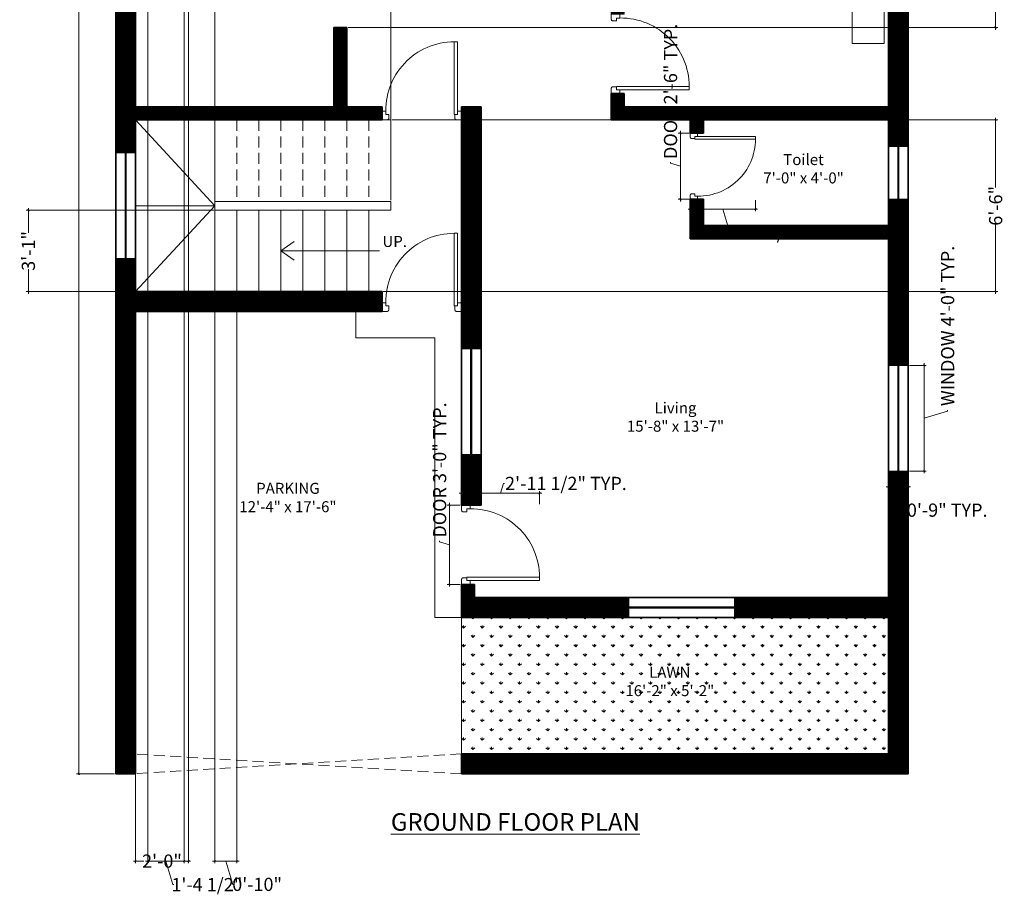
# Model space of a CAD drawing. Units: inches. Extents: x 111008 to 118198, y -138546 to -137723.
# Tile 3 of 4: x 117735 to 118183, y -138546 to -138144. Entities that reach past the tile are written whole.
import ezdxf

# ---------------------------------------------------------------- set-up
doc = ezdxf.new("R2010")
doc.units = ezdxf.units.IN
doc.header["$LTSCALE"] = 20
doc.header["$MEASUREMENT"] = 0
doc.header["$PDMODE"] = 3
doc.linetypes.add('HIDDEN', pattern=[0.375, 0.25, -0.125])
for name, color, linetype, lineweight in [('A-ANNO-DIMS', 2, 'Continuous', 18), ('A-ANNO-TEXT', 7, 'Continuous', 18), ('A-AREA-IDEN', 7, 'Continuous', 18), ('A-DOOR', 181, 'Continuous', 18), ('A-DOOR-HIDN', 1, 'HIDDEN', 13), ('A-FLOR-CASE', 181, 'Continuous', 18), ('A-FLOR-STRS', 181, 'Continuous', 18), ('A-FLOR-STRS-HIDN', 181, 'HIDDEN', 13), ('ele', 6, 'Continuous', 20), ('furn', 181, 'Continuous', 15), ('FURNITURE', 8, 'Continuous', 15), ('L-PVMT', 181, 'Continuous', 18), ('walls', 7, 'Continuous', 35), ('WIN', 181, 'Continuous', 18)]:
    doc.layers.add(name, color=color, linetype=linetype, lineweight=lineweight)
doc.layers.add('A-WALL-PATT', color=251, linetype='Continuous', lineweight=9, true_color=0x636466)
doc.layers.add('L-PLNT-PATT', color=114, linetype='Continuous', lineweight=9, true_color=0x139b48)
doc.styles.add('vn1', font='arial.ttf', dxfattribs={"height": 6})
doc.dimstyles.new('vn1', dxfattribs={"dimtxt": 6, "dimasz": 1, "dimexe": 1, "dimexo": 0.5, "dimgap": 0.25, "dimtad": 0, "dimdec": 1, "dimzin": 3, "dimdsep": 46, "dimlunit": 4, "dimtxsty": 'vn1', "dimblk": 'ARCHTICK', "dimcen": 0, "dimdle": 1, "dimclrd": 8, "dimclre": 8, "dimclrt": 7, "dimadec": 0, "dimazin": 0, "dimtfac": 0.75, "dimtdec": 1, "dimtofl": 0, "dimtmove": 1, "dimatfit": 3, "dimfxl": 1, "dimtolj": 1, "dimtzin": 0, "dimlwd": -1, "dimlwe": -1, "dimarcsym": 0})

# ---------------------------------------------------------------- blocks, each defined once
blk = doc.blocks.new('_ArchTick')
at = {"color": 0, "linetype": 'ByBlock', "const_width": 0.15}
blk.add_lwpolyline([(-0.5, -0.5), (0.5, 0.5)], dxfattribs=at)
blk = doc.blocks.new('*D4')
at = {"layer": 'A-ANNO-DIMS', "color": 0, "transparency": 16777216}
for p, q in [((117778.41, -137766.56), (117761.13, -137766.56)), ((117762.13, -137766.06), (117762.13, -138115.99)), ((117762.13, -138487.06), (117762.13, -138137.13)), ((117778.41, -138486.56), (117761.13, -138486.56))]:
    blk.add_line(p, q, dxfattribs=at)
at = {"layer": 'Defpoints', "color": 0, "transparency": 16777216}
for p in [(117762.13, -137766.56), (117778.91, -137766.56), (117778.91, -138486.56)]:
    blk.add_point(p, dxfattribs=at)
at = {"layer": 'A-ANNO-DIMS', "color": 0, "transparency": 16777216}
for p, rotation in [((117762.13, -137766.56), 90), ((117762.13, -138486.56), 270)]:
    blk.add_blockref('_ArchTick', p, dxfattribs=dict(at, rotation=rotation))
at = {"layer": 'A-ANNO-DIMS', "color": 0, "transparency": 16777216, "insert": (117762.13, -138126.56), "char_height": 6, "attachment_point": 5, "rotation": 90, "style": 'vn1'}
blk.add_mtext('\\A1;60\'-0"', dxfattribs=at)
blk = doc.blocks.new('39 door')
at = {"layer": 'ele'}
blk.add_lwpolyline([(-17.62, 38.46), (-17.62, 2.69), (-16, 2.69), (-16, 38.46)], close=True, dxfattribs=at)
at = {"layer": 'furn'}
for points in [[(-16.87, 0), (-19.5, 0), (-19.5, 0), (-19.5, 4.31), (-17.62, 4.31), (-17.62, 2.69), (-16.27, 2.69), (-16.27, 0.6), (-16.42, 0.6), (-16.42, 0.45, -0.414214), (-16.72, 0.15), (-16.87, 0.15)], [(16.87, 0), (19.5, 0), (19.5, 0), (19.5, 4.31), (17.62, 4.31), (17.62, 2.69), (16.27, 2.69), (16.27, 0.6), (16.42, 0.6), (16.42, 0.45, 0.414214), (16.72, 0.15), (16.87, 0.15)]]:
    blk.add_lwpolyline(points, format="xyb", close=True, dxfattribs=at)
at = {"layer": 'WIN', "ltscale": 0.25}
blk.add_arc((-16.03, 4.75), 33.71, 356.5003, 89.9437, dxfattribs=at)
blk = doc.blocks.new('WIN-48IN')
at = {"ltscale": 0.5}
for p, q in [((0, 48), (0, 0)), ((9, 48), (9, 0))]:
    blk.add_line(p, q, dxfattribs=at)
for p, q in [((0, 48), (9, 48)), ((0, 0), (9, 0))]:
    blk.add_line(p, q)
at = {"ltscale": 0.5, "const_width": 1}
blk.add_lwpolyline([(4.49, 48), (4.49, 0)], dxfattribs=at)
blk = doc.blocks.new('WIN-24IN')
at = {"ltscale": 0.5}
for p, q in [((0, 24), (0, 0)), ((9, 24), (9, 0))]:
    blk.add_line(p, q, dxfattribs=at)
for p, q in [((0, 24), (9, 24)), ((0, 0), (9, 0))]:
    blk.add_line(p, q)
at = {"ltscale": 0.5, "const_width": 1}
blk.add_lwpolyline([(4.49, 24), (4.49, 0)], dxfattribs=at)
blk = doc.blocks.new('BEDSIDE-TABLE')
blk.add_lwpolyline([(0, 16.95), (0, 0), (14.43, 0), (14.43, 16.95)], close=True)
blk = doc.blocks.new('*D11')
at = {"layer": 'A-ANNO-DIMS', "color": 8, "transparency": 16777216}
for p, q in [((117930.51, -138401.56), (117930.51, -138363.56)), ((117935.41, -138364.56), (117929.51, -138364.56)), ((117926.03, -138381.21), (117926.03, -138380.71)), ((117930.51, -138382.56), (117926.03, -138381.21)), ((117935.41, -138400.56), (117929.51, -138400.56))]:
    blk.add_line(p, q, dxfattribs=at)
at = {"layer": 'Defpoints', "color": 0, "transparency": 16777216}
for p in [(117930.51, -138364.56), (117935.91, -138364.56), (117935.91, -138400.56)]:
    blk.add_point(p, dxfattribs=at)
at = {"layer": 'A-ANNO-DIMS', "color": 8, "transparency": 16777216}
for p, rotation in [((117930.51, -138364.56), 90), ((117930.51, -138400.56), 270)]:
    blk.add_blockref('_ArchTick', p, dxfattribs=dict(at, rotation=rotation))
at = {"layer": 'A-ANNO-DIMS', "color": 7, "transparency": 16777216, "insert": (117926.03, -138348.59), "char_height": 6, "attachment_point": 5, "rotation": 90, "style": 'vn1'}
blk.add_mtext('\\A1;DOOR 3\'-0" TYP.', dxfattribs=at)
blk = doc.blocks.new('*D12')
at = {"layer": 'A-ANNO-DIMS', "color": 8, "transparency": 16777216}
for p, q in [((117953.66, -138359.16), (117955, -138354.68)), ((117955, -138354.68), (117955.5, -138354.68)), ((117934.91, -138359.16), (117972.41, -138359.16)), ((117935.91, -138364.06), (117935.91, -138358.16)), ((117971.41, -138364.06), (117971.41, -138358.16))]:
    blk.add_line(p, q, dxfattribs=at)
at = {"layer": 'Defpoints', "color": 0, "transparency": 16777216}
for p in [(117971.41, -138359.16), (117935.91, -138364.56), (117971.41, -138364.56)]:
    blk.add_point(p, dxfattribs=at)
at = {"layer": 'A-ANNO-DIMS', "color": 8, "transparency": 16777216, "rotation": 180}
blk.add_blockref('_ArchTick', (117935.91, -138359.16), dxfattribs=at)
at = {"layer": 'A-ANNO-DIMS', "color": 8, "transparency": 16777216}
blk.add_blockref('_ArchTick', (117971.41, -138359.16), dxfattribs=at)
at = {"layer": 'A-ANNO-DIMS', "color": 7, "transparency": 16777216, "insert": (117983.41, -138354.68), "char_height": 6, "attachment_point": 5, "style": 'vn1'}
blk.add_mtext('\\A1;2\'-11 1/2" TYP.', dxfattribs=at)
blk = doc.blocks.new('*D13')
at = {"layer": 'A-ANNO-DIMS', "color": 8, "transparency": 16777216}
for p, q in [((118039.41, -138195.56), (118034.41, -138195.55)), ((118035.41, -138194.55), (118035.39, -138226.55)), ((118030.92, -138209.21), (118030.92, -138208.71)), ((118035.4, -138210.55), (118030.92, -138209.21)), ((118039.39, -138225.56), (118034.39, -138225.55))]:
    blk.add_line(p, q, dxfattribs=at)
at = {"layer": 'Defpoints', "color": 0, "transparency": 16777216}
for p in [(118039.91, -138195.56), (118035.39, -138225.55), (118039.89, -138225.56)]:
    blk.add_point(p, dxfattribs=at)
at = {"layer": 'A-ANNO-DIMS', "color": 8, "transparency": 16777216}
for p, rotation in [((118035.41, -138195.55), 89.96632877380524), ((118035.39, -138225.55), 269.9663287738052)]:
    blk.add_blockref('_ArchTick', p, dxfattribs=dict(at, rotation=rotation))
at = {"layer": 'A-ANNO-DIMS', "color": 7, "transparency": 16777216, "insert": (118030.94, -138176.58), "char_height": 6, "attachment_point": 5, "rotation": 89.9663, "style": 'vn1'}
blk.add_mtext('\\A1;DOOR 2\'-6" TYP.', dxfattribs=at)
blk = doc.blocks.new('*D14')
at = {"layer": 'A-ANNO-DIMS', "color": 8, "transparency": 16777216}
for p, q in [((118038.89, -138230.06), (118070.47, -138230.08)), ((118039.89, -138226.06), (118039.89, -138231.06)), ((118054.68, -138230.07), (118057.88, -138240.75)), ((118069.48, -138226.07), (118069.47, -138231.07)), ((118057.88, -138240.75), (118058.38, -138240.75))]:
    blk.add_line(p, q, dxfattribs=at)
at = {"layer": 'Defpoints', "color": 0, "transparency": 16777216}
for p in [(118039.89, -138225.56), (118069.48, -138225.57), (118069.47, -138230.07)]:
    blk.add_point(p, dxfattribs=at)
at = {"layer": 'A-ANNO-DIMS', "color": 8, "transparency": 16777216}
for p, rotation in [((118039.89, -138230.06), 179.9663287737755), ((118069.47, -138230.07), 359.9663287737755)]:
    blk.add_blockref('_ArchTick', p, dxfattribs=dict(at, rotation=rotation))
at = {"layer": 'A-ANNO-DIMS', "color": 7, "transparency": 16777216, "insert": (118083.96, -138240.77), "char_height": 6, "attachment_point": 5, "rotation": 359.9663, "style": 'vn1'}
blk.add_mtext('\\A1;2\'-5 1/2" TYP.', dxfattribs=at)
blk = doc.blocks.new('*D15')
at = {"layer": 'A-ANNO-DIMS', "color": 8, "transparency": 16777216}
for p, q in [((118139.41, -138301.06), (118147.11, -138301.06)), ((118146.11, -138350.06), (118146.11, -138300.06)), ((118146.11, -138325.06), (118156.8, -138321.85)), ((118156.8, -138321.85), (118156.8, -138321.35)), ((118139.41, -138349.06), (118147.11, -138349.06))]:
    blk.add_line(p, q, dxfattribs=at)
at = {"layer": 'Defpoints', "color": 0, "transparency": 16777216}
for p in [(118138.91, -138301.06), (118146.11, -138301.06), (118138.91, -138349.06)]:
    blk.add_point(p, dxfattribs=at)
at = {"layer": 'A-ANNO-DIMS', "color": 8, "transparency": 16777216}
for p, rotation in [((118146.11, -138301.06), 90), ((118146.11, -138349.06), 270)]:
    blk.add_blockref('_ArchTick', p, dxfattribs=dict(at, rotation=rotation))
at = {"layer": 'A-ANNO-DIMS', "color": 7, "transparency": 16777216, "insert": (118156.8, -138283.14), "char_height": 6, "attachment_point": 5, "rotation": 90, "style": 'vn1'}
blk.add_mtext('\\A1;WINDOW 4\'-0" TYP.', dxfattribs=at)
blk = doc.blocks.new('*D16')
at = {"layer": 'A-ANNO-DIMS', "color": 8, "transparency": 16777216}
for p, q in [((118129.91, -138349.56), (118129.91, -138357.26)), ((118138.91, -138349.56), (118138.91, -138357.26)), ((118128.91, -138356.26), (118139.91, -138356.26)), ((118134.41, -138356.26), (118137.58, -138366.82)), ((118137.58, -138366.82), (118138.08, -138366.82))]:
    blk.add_line(p, q, dxfattribs=at)
at = {"layer": 'Defpoints', "color": 0, "transparency": 16777216}
for p in [(118129.91, -138349.06), (118138.91, -138349.06), (118138.91, -138356.26)]:
    blk.add_point(p, dxfattribs=at)
at = {"layer": 'A-ANNO-DIMS', "color": 8, "transparency": 16777216, "rotation": 180}
blk.add_blockref('_ArchTick', (118129.91, -138356.26), dxfattribs=at)
at = {"layer": 'A-ANNO-DIMS', "color": 8, "transparency": 16777216}
blk.add_blockref('_ArchTick', (118138.91, -138356.26), dxfattribs=at)
at = {"layer": 'A-ANNO-DIMS', "color": 7, "transparency": 16777216, "insert": (118156.61, -138366.82), "char_height": 6, "attachment_point": 5, "style": 'vn1'}
blk.add_mtext('\\A1;0\'-9" TYP.', dxfattribs=at)
blk = doc.blocks.new('*D25')
at = {"layer": 'A-ANNO-DIMS', "color": 8, "transparency": 16777216}
for p, q in [((117787.91, -138184.06), (117787.91, -138527.26)), ((117811.91, -138184.06), (117811.91, -138527.26)), ((117786.91, -138526.26), (117791.63, -138526.26)), ((117812.91, -138526.26), (117808.18, -138526.26))]:
    blk.add_line(p, q, dxfattribs=at)
at = {"layer": 'Defpoints', "color": 0, "transparency": 16777216}
for p in [(117787.91, -138183.56), (117811.91, -138183.56), (117811.91, -138526.26)]:
    blk.add_point(p, dxfattribs=at)
at = {"layer": 'A-ANNO-DIMS', "color": 8, "transparency": 16777216, "rotation": 180}
blk.add_blockref('_ArchTick', (117787.91, -138526.26), dxfattribs=at)
at = {"layer": 'A-ANNO-DIMS', "color": 8, "transparency": 16777216}
blk.add_blockref('_ArchTick', (117811.91, -138526.26), dxfattribs=at)
at = {"layer": 'A-ANNO-DIMS', "color": 7, "transparency": 16777216, "insert": (117799.91, -138526.26), "char_height": 6, "attachment_point": 5, "style": 'vn1'}
blk.add_mtext('\\A1;2\'-0"', dxfattribs=at)
blk = doc.blocks.new('*D26')
at = {"layer": 'A-ANNO-DIMS', "color": 8, "transparency": 16777216}
for p, q in [((117884.41, -138063.56), (118179.61, -138063.56)), ((118178.61, -138062.56), (118178.61, -138097.36)), ((118178.61, -138148.56), (118178.61, -138113.76)), ((117884.41, -138147.56), (118179.61, -138147.56))]:
    blk.add_line(p, q, dxfattribs=at)
at = {"layer": 'Defpoints', "color": 0, "transparency": 16777216}
for p in [(117883.91, -138063.56), (117883.91, -138147.56), (118178.61, -138147.56)]:
    blk.add_point(p, dxfattribs=at)
at = {"layer": 'A-ANNO-DIMS', "color": 8, "transparency": 16777216}
for p, rotation in [((118178.61, -138063.56), 90), ((118178.61, -138147.56), 270)]:
    blk.add_blockref('_ArchTick', p, dxfattribs=dict(at, rotation=rotation))
at = {"layer": 'A-ANNO-DIMS', "color": 7, "transparency": 16777216, "insert": (118178.61, -138105.56), "char_height": 6, "attachment_point": 5, "rotation": 90, "style": 'vn1'}
blk.add_mtext('\\A1;7\'-0"', dxfattribs=at)
blk = doc.blocks.new('*D27')
at = {"layer": 'A-ANNO-DIMS', "color": 8, "transparency": 16777216}
for p, q in [((117793.41, -138135.94), (117793.41, -138527.26)), ((117809.91, -138135.94), (117809.91, -138527.26)), ((117792.41, -138526.26), (117810.91, -138526.26)), ((117801.66, -138526.26), (117804.86, -138536.94)), ((117804.86, -138536.94), (117805.36, -138536.94))]:
    blk.add_line(p, q, dxfattribs=at)
at = {"layer": 'Defpoints', "color": 0, "transparency": 16777216}
for p in [(117793.41, -138135.44), (117809.91, -138135.44), (117809.91, -138526.26)]:
    blk.add_point(p, dxfattribs=at)
at = {"layer": 'A-ANNO-DIMS', "color": 8, "transparency": 16777216, "rotation": 180}
blk.add_blockref('_ArchTick', (117793.41, -138526.26), dxfattribs=at)
at = {"layer": 'A-ANNO-DIMS', "color": 8, "transparency": 16777216}
blk.add_blockref('_ArchTick', (117809.91, -138526.26), dxfattribs=at)
at = {"layer": 'A-ANNO-DIMS', "color": 7, "transparency": 16777216, "insert": (117820.29, -138536.94), "char_height": 6, "attachment_point": 5, "style": 'vn1'}
blk.add_mtext('\\A1;1\'-4 1/2"', dxfattribs=at)
blk = doc.blocks.new('*D31')
at = {"layer": 'A-ANNO-DIMS', "color": 8, "transparency": 16777216}
for p, q in [((117823.91, -138268.06), (117823.91, -138527.26)), ((117833.91, -138268.06), (117833.91, -138527.26)), ((117822.91, -138526.26), (117834.91, -138526.26)), ((117828.91, -138526.26), (117832.08, -138536.82)), ((117832.08, -138536.82), (117832.58, -138536.82))]:
    blk.add_line(p, q, dxfattribs=at)
at = {"layer": 'Defpoints', "color": 0, "transparency": 16777216}
for p in [(117823.91, -138267.56), (117833.91, -138267.56), (117833.91, -138526.26)]:
    blk.add_point(p, dxfattribs=at)
at = {"layer": 'A-ANNO-DIMS', "color": 8, "transparency": 16777216, "rotation": 180}
blk.add_blockref('_ArchTick', (117823.91, -138526.26), dxfattribs=at)
at = {"layer": 'A-ANNO-DIMS', "color": 8, "transparency": 16777216}
blk.add_blockref('_ArchTick', (117833.91, -138526.26), dxfattribs=at)
at = {"layer": 'A-ANNO-DIMS', "color": 7, "transparency": 16777216, "insert": (117843.13, -138536.82), "char_height": 6, "attachment_point": 5, "style": 'vn1'}
blk.add_mtext('\\A1;0\'-10"', dxfattribs=at)
blk = doc.blocks.new('*D32')
at = {"layer": 'A-ANNO-DIMS', "color": 8, "transparency": 16777216}
for p, q in [((117739.21, -138229.56), (117739.21, -138240.83)), ((117823.41, -138230.56), (117738.21, -138230.56)), ((117739.21, -138268.56), (117739.21, -138257.28)), ((117823.41, -138267.56), (117738.21, -138267.56))]:
    blk.add_line(p, q, dxfattribs=at)
at = {"layer": 'Defpoints', "color": 0, "transparency": 16777216}
for p in [(117739.21, -138230.56), (117823.91, -138230.56), (117823.91, -138267.56)]:
    blk.add_point(p, dxfattribs=at)
at = {"layer": 'A-ANNO-DIMS', "color": 8, "transparency": 16777216}
for p, rotation in [((117739.21, -138230.56), 90), ((117739.21, -138267.56), 270)]:
    blk.add_blockref('_ArchTick', p, dxfattribs=dict(at, rotation=rotation))
at = {"layer": 'A-ANNO-DIMS', "color": 7, "transparency": 16777216, "insert": (117739.21, -138249.06), "char_height": 6, "attachment_point": 5, "rotation": 90, "style": 'vn1'}
blk.add_mtext('\\A1;3\'-1"', dxfattribs=at)
blk = doc.blocks.new('*D33')
at = {"layer": 'A-ANNO-DIMS', "color": 8, "transparency": 16777216}
for p, q in [((117786.91, -137726.86), (117797.68, -137726.86)), ((117787.91, -138228.06), (117787.91, -137725.86)), ((117824.91, -137726.86), (117814.13, -137726.86)), ((117823.91, -138228.06), (117823.91, -137725.86))]:
    blk.add_line(p, q, dxfattribs=at)
at = {"layer": 'Defpoints', "color": 0, "transparency": 16777216}
for p in [(117823.91, -137726.86), (117787.91, -138228.56), (117823.91, -138228.56)]:
    blk.add_point(p, dxfattribs=at)
at = {"layer": 'A-ANNO-DIMS', "color": 8, "transparency": 16777216, "rotation": 180}
blk.add_blockref('_ArchTick', (117787.91, -137726.86), dxfattribs=at)
at = {"layer": 'A-ANNO-DIMS', "color": 8, "transparency": 16777216}
blk.add_blockref('_ArchTick', (117823.91, -137726.86), dxfattribs=at)
at = {"layer": 'A-ANNO-DIMS', "color": 7, "transparency": 16777216, "insert": (117805.91, -137726.86), "char_height": 6, "attachment_point": 5, "style": 'vn1'}
blk.add_mtext('\\A1;3\'-0"', dxfattribs=at)
blk = doc.blocks.new('*D34')
at = {"layer": 'A-ANNO-DIMS', "color": 8, "transparency": 16777216}
for p, q in [((117822.91, -137726.86), (117855.67, -137726.86)), ((117823.91, -138226.06), (117823.91, -137725.86)), ((117904.91, -137726.86), (117872.15, -137726.86)), ((117903.91, -138226.06), (117903.91, -137725.86))]:
    blk.add_line(p, q, dxfattribs=at)
at = {"layer": 'Defpoints', "color": 0, "transparency": 16777216}
for p in [(117903.91, -137726.86), (117823.91, -138226.56), (117903.91, -138226.56)]:
    blk.add_point(p, dxfattribs=at)
at = {"layer": 'A-ANNO-DIMS', "color": 8, "transparency": 16777216, "rotation": 180}
blk.add_blockref('_ArchTick', (117823.91, -137726.86), dxfattribs=at)
at = {"layer": 'A-ANNO-DIMS', "color": 8, "transparency": 16777216}
blk.add_blockref('_ArchTick', (117903.91, -137726.86), dxfattribs=at)
at = {"layer": 'A-ANNO-DIMS', "color": 7, "transparency": 16777216, "insert": (117863.91, -137726.86), "char_height": 6, "attachment_point": 5, "style": 'vn1'}
blk.add_mtext('\\A1;6\'-8"', dxfattribs=at)
blk = doc.blocks.new('*D35')
at = {"layer": 'A-ANNO-DIMS', "color": 8, "transparency": 16777216}
for p, q in [((117904.41, -138189.56), (118179.61, -138189.56)), ((118178.61, -138188.56), (118178.61, -138220.32)), ((118178.61, -138268.56), (118178.61, -138236.8)), ((117900.41, -138267.56), (118179.61, -138267.56))]:
    blk.add_line(p, q, dxfattribs=at)
at = {"layer": 'Defpoints', "color": 0, "transparency": 16777216}
for p in [(117903.91, -138189.56), (118178.61, -138189.56), (117899.91, -138267.56)]:
    blk.add_point(p, dxfattribs=at)
at = {"layer": 'A-ANNO-DIMS', "color": 8, "transparency": 16777216}
for p, rotation in [((118178.61, -138189.56), 90), ((118178.61, -138267.56), 270)]:
    blk.add_blockref('_ArchTick', p, dxfattribs=dict(at, rotation=rotation))
at = {"layer": 'A-ANNO-DIMS', "color": 7, "transparency": 16777216, "insert": (118178.61, -138228.56), "char_height": 6, "attachment_point": 5, "rotation": 90, "style": 'vn1'}
blk.add_mtext('\\A1;6\'-6"', dxfattribs=at)

msp = doc.modelspace()

# ---------------------------------------------------------------- hatches: boundary and pattern name
at = {"layer": 'A-WALL-PATT'}
h = msp.add_hatch(dxfattribs=at)
h.set_pattern_fill('ANSI31', color=256)
h.paths.add_polyline_path([(117829.91, -137766.56), (117778.91, -137766.56), (117778.91, -137919.56), (117787.91, -137919.56), (117787.91, -137865.56), (117826.91, -137865.56), (117826.91, -137859.56), (117787.91, -137859.56), (117787.91, -137775.56), (117829.91, -137775.56)])
h.paths.add_polyline_path([(117865.91, -137766.56), (117853.91, -137766.56), (117853.91, -137775.56), (117859.91, -137775.56), (117859.91, -137859.56), (117856.91, -137859.56), (117856.91, -137865.56), (117868.91, -137865.56), (117868.91, -137861.58), (117868.91, -137859.56), (117865.91, -137859.56)])
h.paths.add_polyline_path([(118099.91, -137766.56), (118051.91, -137766.56), (118051.91, -137859.56), (118048.91, -137859.56), (118048.91, -137865.56), (118060.91, -137865.56), (118060.91, -137862.24), (118060.91, -137859.56), (118057.91, -137859.56), (118057.91, -137775.56), (118099.91, -137775.56)])
h.paths.add_polyline_path([(118138.91, -137766.56), (118123.91, -137766.56), (118123.91, -137775.56), (118129.91, -137775.56), (118129.91, -137859.56), (118090.91, -137859.56), (118090.91, -137865.56), (118129.91, -137865.56), (118129.91, -137919.56), (118138.91, -137919.56)])
h.paths.add_polyline_path([(118138.91, -137967.56), (118129.91, -137967.56), (118129.91, -138021.56), (118003.91, -138021.56), (118003.91, -138141.56), (118007.88, -138141.56), (118009.91, -138141.56), (118009.91, -138027.56), (118129.91, -138027.56), (118129.91, -138081.56), (118138.91, -138081.56)])
h.paths.add_polyline_path([(118012.91, -137861.58), (118012.91, -137859.56), (117904.91, -137859.56), (117904.91, -137865.56), (117960.91, -137865.56), (117960.91, -138021.56), (117954.91, -138021.56), (117954.91, -138027.56), (117967.91, -138027.56), (117967.91, -138023.58), (117967.91, -138021.56), (117966.91, -138021.56), (117966.91, -137865.56), (118012.91, -137865.56)])
h.paths.add_polyline_path([(117787.91, -138027.56), (117877.91, -138027.56), (117877.91, -138063.56), (117883.91, -138063.56), (117883.91, -138027.56), (117918.91, -138027.56), (117918.91, -138023.58), (117918.91, -138021.56), (117787.91, -138021.56), (117787.91, -137967.56), (117778.91, -137967.56), (117778.91, -138081.56), (117787.91, -138081.56)])
h.paths.add_polyline_path([(117787.91, -138129.56), (117778.91, -138129.56), (117778.91, -138204.56), (117787.91, -138204.56), (117787.91, -138189.56), (117899.91, -138189.56), (117899.91, -138185.58), (117899.91, -138183.56), (117883.91, -138183.56), (117883.91, -138147.56), (117877.91, -138147.56), (117877.91, -138183.56), (117787.91, -138183.56)])
h.paths.add_polyline_path([(118138.91, -138129.56), (118129.91, -138129.56), (118129.91, -138183.56), (118009.91, -138183.56), (118009.91, -138177.56), (118003.91, -138177.56), (118003.91, -138189.56), (118039.91, -138189.56), (118039.91, -138195.56), (118045.91, -138195.56), (118045.91, -138189.56), (118129.91, -138189.56), (118129.91, -138201.56), (118138.91, -138201.56)])
h.paths.add_polyline_path([(118138.91, -138225.56), (118129.91, -138225.56), (118129.91, -138237.56), (118045.91, -138237.56), (118045.91, -138225.56), (118043.2, -138225.56), (118043.2, -138225.56), (118039.91, -138225.56), (118039.91, -138243.56), (118129.91, -138243.56), (118129.91, -138301.06), (118138.91, -138301.06)])
h.paths.add_polyline_path([(117944.91, -138183.56), (117935.91, -138183.56), (117935.91, -138293.56), (117944.91, -138293.56)])
h.paths.add_polyline_path([(117899.91, -138267.56), (117787.91, -138267.56), (117787.91, -138252.56), (117778.91, -138252.56), (117778.91, -138486.56), (117787.91, -138486.56), (117787.91, -138276.56), (117899.91, -138276.56), (117899.91, -138272.58)])
h.paths.add_polyline_path([(117944.91, -138341.56), (117935.91, -138341.56), (117935.91, -138364.56), (117939.88, -138364.56), (117944.91, -138364.56)])
h.paths.add_polyline_path([(118011.91, -138406.56), (117941.91, -138406.56), (117941.91, -138400.56), (117935.91, -138400.56), (117935.91, -138415.56), (118011.91, -138415.56)], flags=17)
h.paths.add_polyline_path([(118138.91, -138349.06), (118129.91, -138349.06), (118129.91, -138406.56), (118059.91, -138406.56), (118059.91, -138415.56), (118129.91, -138415.56), (118129.91, -138477.56), (117935.91, -138477.56), (117935.91, -138486.56), (118138.91, -138486.56)])
at = {"layer": 'L-PLNT-PATT'}
h = msp.add_hatch(dxfattribs=at)
h.set_pattern_fill('GRASS', color=256, scale=6)
h.paths.add_polyline_path([(118129.91, -138415.56), (117935.91, -138415.56), (117935.91, -138477.56), (118129.91, -138477.56)])

# ---------------------------------------------------------------- linework, layer by layer
at = {"layer": 'A-DOOR-HIDN'}
for p, q in [((117935.91, -138486.56), (117787.91, -138477.56)), ((117935.91, -138477.56), (117787.91, -138486.56))]:
    msp.add_line(p, q, dxfattribs=at)
at = {"layer": 'A-FLOR-CASE'}
msp.add_line((117811.91, -138051.56), (117811.91, -138183.56), dxfattribs=at)
at = {"layer": 'A-FLOR-STRS'}
for p, q in [((117823.91, -138228.56), (117787.91, -138189.56)), ((117823.91, -138228.56), (117787.91, -138228.56)), ((117823.91, -138228.56), (117787.91, -138267.56)), ((117823.91, -138226.56), (117903.91, -138226.56)), ((117823.91, -138226.56), (117823.91, -138230.56)), ((117823.91, -138230.56), (117903.91, -138230.56)), ((117823.91, -138230.56), (117823.91, -138267.56)), ((117833.91, -138230.56), (117833.91, -138267.56)), ((117843.91, -138230.56), (117843.91, -138267.56)), ((117853.91, -138230.56), (117853.91, -138267.56)), ((117863.91, -138230.56), (117863.91, -138267.56)), ((117873.91, -138230.56), (117873.91, -138267.56)), ((117883.91, -138230.56), (117883.91, -138267.56)), ((117893.91, -138230.56), (117893.91, -138267.56))]:
    msp.add_line(p, q, dxfattribs=at)
at = {"layer": 'A-FLOR-STRS-HIDN'}
for p, q in [((117823.91, -138189.56), (117823.91, -138226.56)), ((117833.91, -138189.56), (117833.91, -138226.56)), ((117843.91, -138189.56), (117843.91, -138226.56)), ((117853.91, -138189.56), (117853.91, -138226.56)), ((117863.91, -138189.56), (117863.91, -138226.56)), ((117873.91, -138189.56), (117873.91, -138226.56)), ((117883.91, -138189.56), (117883.91, -138226.56)), ((117893.91, -138189.56), (117893.91, -138226.56)), ((117899.91, -138189.56), (117903.91, -138189.56)), ((117903.91, -138189.56), (117903.91, -138226.56)), ((117903.91, -138226.56), (117903.91, -138230.56))]:
    msp.add_line(p, q, dxfattribs=at)
at = {"layer": 'L-PVMT'}
for p, q in [((117887.91, -138276.56), (117887.91, -138288.56)), ((117923.91, -138288.56), (117887.91, -138288.56)), ((117923.91, -138288.56), (117923.91, -138415.56)), ((117935.91, -138415.56), (117923.91, -138415.56)), ((117935.91, -138415.56), (117935.91, -138477.56))]:
    msp.add_line(p, q, dxfattribs=at)
at = {"layer": 'walls'}
for p, q in [((117787.91, -138027.56), (117787.91, -138183.56)), ((118129.91, -138183.56), (118129.91, -138027.56)), ((117883.91, -138147.56), (117877.91, -138147.56)), ((117877.91, -138147.56), (117877.91, -138183.56)), ((117883.91, -138147.56), (117883.91, -138183.56)), ((118003.91, -138189.56), (118003.91, -138177.56)), ((118009.91, -138177.56), (118003.91, -138177.56)), ((118009.91, -138183.56), (118009.91, -138177.56)), ((117877.91, -138183.56), (117787.91, -138183.56)), ((117899.91, -138183.56), (117883.91, -138183.56)), ((117899.91, -138183.56), (117899.91, -138189.56)), ((117935.91, -138183.56), (117935.91, -138364.56)), ((117944.91, -138183.56), (117935.91, -138183.56)), ((117944.91, -138183.56), (117944.91, -138364.56)), ((118129.91, -138183.56), (118009.91, -138183.56)), ((117899.91, -138189.56), (117787.91, -138189.56)), ((117787.91, -138189.56), (117787.91, -138267.56)), ((118039.91, -138189.56), (118003.91, -138189.56)), ((118039.91, -138195.56), (118039.91, -138189.56)), ((118129.91, -138189.56), (118045.91, -138189.56)), ((118045.91, -138195.56), (118045.91, -138189.56)), ((118129.91, -138237.56), (118129.91, -138189.56)), ((118045.91, -138195.56), (118039.91, -138195.56)), ((118039.91, -138243.56), (118039.91, -138225.56)), ((118045.91, -138225.56), (118039.91, -138225.56)), ((118045.91, -138237.56), (118045.91, -138225.56)), ((118129.91, -138237.56), (118045.91, -138237.56)), ((118129.91, -138243.56), (118039.91, -138243.56)), ((118129.91, -138406.56), (118129.91, -138243.56)), ((117899.91, -138267.56), (117787.91, -138267.56)), ((117899.91, -138267.56), (117899.91, -138276.56)), ((117899.91, -138276.56), (117787.91, -138276.56)), ((117787.91, -138276.56), (117787.91, -138486.56)), ((117935.91, -138364.56), (117944.91, -138364.56)), ((117935.91, -138400.56), (117941.91, -138400.56)), ((117935.91, -138400.56), (117935.91, -138415.56)), ((117941.91, -138400.56), (117941.91, -138406.56)), ((117941.91, -138406.56), (118129.91, -138406.56)), ((117935.91, -138415.56), (118129.91, -138415.56)), ((118129.91, -138477.56), (118129.91, -138415.56)), ((117935.91, -138477.56), (118129.91, -138477.56)), ((117935.91, -138477.56), (117935.91, -138486.56))]:
    msp.add_line(p, q, dxfattribs=at)
for points in [[(117865.91, -137766.56), (117778.91, -137766.56), (117778.91, -138486.56), (117787.91, -138486.56)], [(117935.91, -138486.56), (118138.91, -138486.56), (118138.91, -137766.56), (118051.91, -137766.56)]]:
    msp.add_lwpolyline(points, dxfattribs=at)

# ---------------------------------------------------------------- block references
at = {"layer": 'A-DOOR', "ltscale": 0.15}
for p, xscale, yscale, zscale, rotation in [((118003.91, -138159.56), -0.9230769230771328, 0.9230769230771328, 0.9230769230771328, 270), ((118039.9, -138210.56), 0.7692306364006699, 0.7692306364006699, 0.7692306364006699, 269.9663287737836), ((117935.91, -138382.56), -0.9230769230771328, 0.9230769230771328, 0.9230769230771328, 270)]:
    msp.add_blockref('39 door', p, dxfattribs=dict(at, xscale=xscale, yscale=yscale, zscale=zscale, rotation=rotation))
at = {"layer": 'A-DOOR', "ltscale": 0.15, "xscale": -0.9230769230771328, "yscale": 0.9230769230771328, "zscale": 0.9230769230771328}
for p in [(117917.91, -138189.56), (117917.91, -138276.56)]:
    msp.add_blockref('39 door', p, dxfattribs=at)
at = {"layer": 'FURNITURE', "extrusion": (0, 0, -1), "zscale": -1}
msp.add_blockref('BEDSIDE-TABLE', (-118127.91, -138154.88), dxfattribs=at)
at = {"layer": 'WIN'}
for name, p in [('WIN-24IN', (118129.91, -138225.56)), ('WIN-48IN', (117778.91, -138252.56)), ('WIN-48IN', (117935.91, -138341.56)), ('WIN-48IN', (118129.91, -138349.06))]:
    msp.add_blockref(name, p, dxfattribs=at)
at = {"layer": 'WIN', "rotation": 269.9999999997734}
msp.add_blockref('WIN-48IN', (118011.91, -138406.56), dxfattribs=at)

# ---------------------------------------------------------------- texts
at = {"layer": 'A-ANNO-TEXT', "attachment_point": 1, "style": 'vn1'}
for s, width, insert, char_height in [('\\pxqc;UP.', 54.6246, (117878.31, -138242.26), 5), ('\\pxqc;{\\fArial|b1|i0|c0|p34;\\LGROUND FLOOR PLAN}', 145.6165, (117887.65, -138504.47), 8)]:
    msp.add_mtext_dynamic_manual_height_columns(s, width=width, gutter_width=30, heights=[0], dxfattribs=dict(at, insert=insert, char_height=char_height))
at = {"layer": 'A-AREA-IDEN', "char_height": 5, "attachment_point": 1, "style": 'vn1'}
for s, insert in [('\\pxqc;Toilet\\P7\'-0" x 4\'-0"', (118064.03, -138205.06)), ('\\pxqc;Living\\P15\'-8" x 13\'-7"', (118005.88, -138317.85)), ('\\pxqc;PARKING\\P12\'-4" x 17\'-6"', (117829.81, -138354.41)), ('\\pxqc;LAWN\\P16\'-2" x 5\'-2"', (118003.29, -138437.99))]:
    msp.add_mtext_dynamic_manual_height_columns(s, width=54.6246, gutter_width=30, heights=[0], dxfattribs=dict(at, insert=insert))

# ---------------------------------------------------------------- dimensions: what is measured, and where the dimension line sits
at = {"layer": 'A-ANNO-DIMS'}
for base, p1, p2, picture, middle in [((117823.91, -137726.86), (117787.91, -138228.56), (117823.91, -138228.56), '*D33', (117805.91, -137726.86)), ((117903.91, -137726.86), (117823.91, -138226.56), (117903.91, -138226.56), '*D34', (117863.91, -137726.86)), ((117809.91, -138526.26), (117793.41, -138135.44), (117809.91, -138135.44), '*D27', (117805.61, -138536.94)), ((117811.91, -138526.26), (117787.91, -138183.56), (117811.91, -138183.56), '*D25', (117799.91, -138526.26)), ((117833.91, -138526.26), (117823.91, -138267.56), (117833.91, -138267.56), '*D31', (117832.83, -138536.82))]:
    dim = msp.add_linear_dim(base=base, p1=p1, p2=p2, dimstyle='vn1', override={"dimdec": 1, "dimlfac": 1, "dimrnd": 0, "dimzin": 1, "dimdsep": 46, "dimlunit": 4, "dimfrac": 2}, dxfattribs=at)
    dim.commit()
    dim.dimension.update_dxf_attribs({"geometry": picture, "text_midpoint": middle})
for base, p1, p2, override, picture, middle in [((117762.13, -137766.56), (117778.91, -138486.56), (117778.91, -137766.56), {"dimdle": 0.5, "dimclrd": 0, "dimclre": 0, "dimclrt": 0}, '*D4', (117762.13, -138126.56)), ((118178.61, -138147.56), (117883.91, -138063.56), (117883.91, -138147.56), {"dimdec": 1, "dimlfac": 1, "dimrnd": 0, "dimzin": 1, "dimdsep": 46, "dimlunit": 4, "dimfrac": 2}, '*D26', (118178.61, -138105.56)), ((118178.61, -138189.56), (117899.91, -138267.56), (117903.91, -138189.56), {"dimdec": 1, "dimlfac": 1, "dimrnd": 0, "dimzin": 1, "dimdsep": 46, "dimlunit": 4, "dimfrac": 2}, '*D35', (118178.61, -138228.56)), ((117739.21, -138230.56), (117823.91, -138267.56), (117823.91, -138230.56), {"dimdec": 1, "dimlfac": 1, "dimrnd": 0, "dimzin": 1, "dimdsep": 46, "dimlunit": 4, "dimfrac": 2}, '*D32', (117739.21, -138249.06))]:
    dim = msp.add_linear_dim(base=base, p1=p1, p2=p2, angle=90, dimstyle='vn1', override=override, dxfattribs=at)
    dim.commit()
    dim.dimension.update_dxf_attribs({"geometry": picture, "text_midpoint": middle})
for base, p1, p2, angle, text, picture, middle in [((118035.39, -138225.55), (118039.91, -138195.56), (118039.89, -138225.56), 269.9663, 'DOOR <> TYP.', '*D13', (118030.92, -138208.46)), ((118069.47, -138230.07), (118039.89, -138225.56), (118069.48, -138225.57), 359.9663, '<> TYP.', '*D14', (118058.63, -138240.75)), ((118146.11, -138301.06), (118138.91, -138349.06), (118138.91, -138301.06), 90, 'WINDOW <> TYP.', '*D15', (118156.8, -138321.1)), ((117930.51, -138364.56), (117935.91, -138400.56), (117935.91, -138364.56), 90, 'DOOR <> TYP.', '*D11', (117926.03, -138380.46))]:
    dim = msp.add_linear_dim(base=base, p1=p1, p2=p2, angle=angle, text=text, dimstyle='vn1', override={"dimdec": 1, "dimlfac": 1, "dimrnd": 0, "dimzin": 1, "dimdsep": 46, "dimlunit": 4, "dimfrac": 2}, dxfattribs=at)
    dim.commit()
    dim.dimension.update_dxf_attribs({"geometry": picture, "text_midpoint": middle})
for base, p1, p2, picture, middle in [((117971.41, -138359.16), (117935.91, -138364.56), (117971.41, -138364.56), '*D12', (117955.75, -138354.68)), ((118138.91, -138356.26), (118129.91, -138349.06), (118138.91, -138349.06), '*D16', (118138.33, -138366.82))]:
    dim = msp.add_linear_dim(base=base, p1=p1, p2=p2, text='<> TYP.', dimstyle='vn1', override={"dimdec": 1, "dimlfac": 1, "dimrnd": 0, "dimzin": 1, "dimdsep": 46, "dimlunit": 4, "dimfrac": 2}, dxfattribs=at)
    dim.commit()
    dim.dimension.update_dxf_attribs({"geometry": picture, "text_midpoint": middle})

# ---------------------------------------------------------------- leaders
at = {"layer": 'A-ANNO-TEXT'}
msp.add_leader([(117853.91, -138249.06), (117898.72, -138249.06)], dimstyle='vn1', override={"dimasz": 6, "dimgap": 0.25, "dimtad": 0, "dimdle": 0.5, "dimclrt": 6, "dimldrblk": 'Open90'}, dxfattribs=at)

doc.saveas('drawing.dxf')
